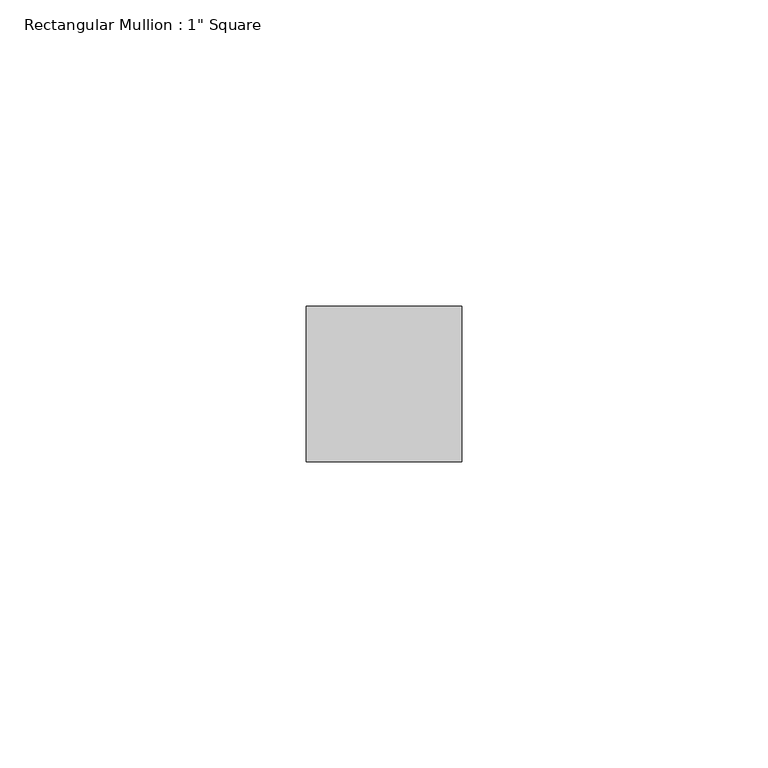
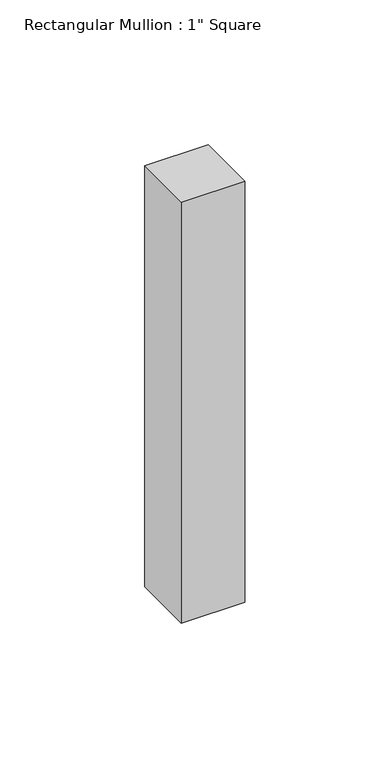
"""IFC4 building model written with IfcOpenShell, lengths in millimetres: member geometry."""

from ifc_helpers import new_model, si_unit, frame, origin, place, context, project, spatial, polyline, outline, extrude, source, transform, mapped, element, save


def member_a0100b10(model_context):
    return source(origin(), model_context, "Body", "SweptSolid", [
        extrude(outline(polyline([(12.7, 12.7), (12.7, -12.7), (-12.7, -12.7), (-12.7, 12.7), (12.7, 12.7)])), frame((0.0, 0.0, -177.8), z_axis=(0.0, 0.0, 1.0), x_axis=(1.0, 0.0, 0.0)), (0.0, 0.0, 1.0), 177.8),
    ])


if __name__ == "__main__":
    model = new_model("IFC4")
    model_context = context("Model", 3, world=origin())
    ifc_project = project(units=[si_unit("LENGTHUNIT", "METRE", prefix="MILLI")], contexts=[model_context])
    site = spatial("IfcSite", under=ifc_project)
    building = spatial("IfcBuilding", under=site)
    placement = place(None, origin())
    member_shape = member_a0100b10(model_context)
    element("IfcMember", 1, ObjectType="Rectangular Mullion : 1\" Square", at=placement, inside=building, context=model_context, shape_type="MappedRepresentation", body=[
        mapped(member_shape, transform((0.0, 0.0, 0.0), x_axis=(1.0, 0.0, 0.0), y_axis=(0.0, 1.0, 0.0), z_axis=(0.0, 0.0, 1.0))),
    ])
    save(model, "model.ifc")

# Revit data of these elements
# Type "Rectangular Mullion : 1\" Square"
#   built-in parameter 1007304 = 0.0833333 (stored number, unit not read)
#   built-in parameter 1007301 = 0.0416667 (stored number, unit not read)
#   built-in parameter 1007300 = 0.0416667 (stored number, unit not read)
